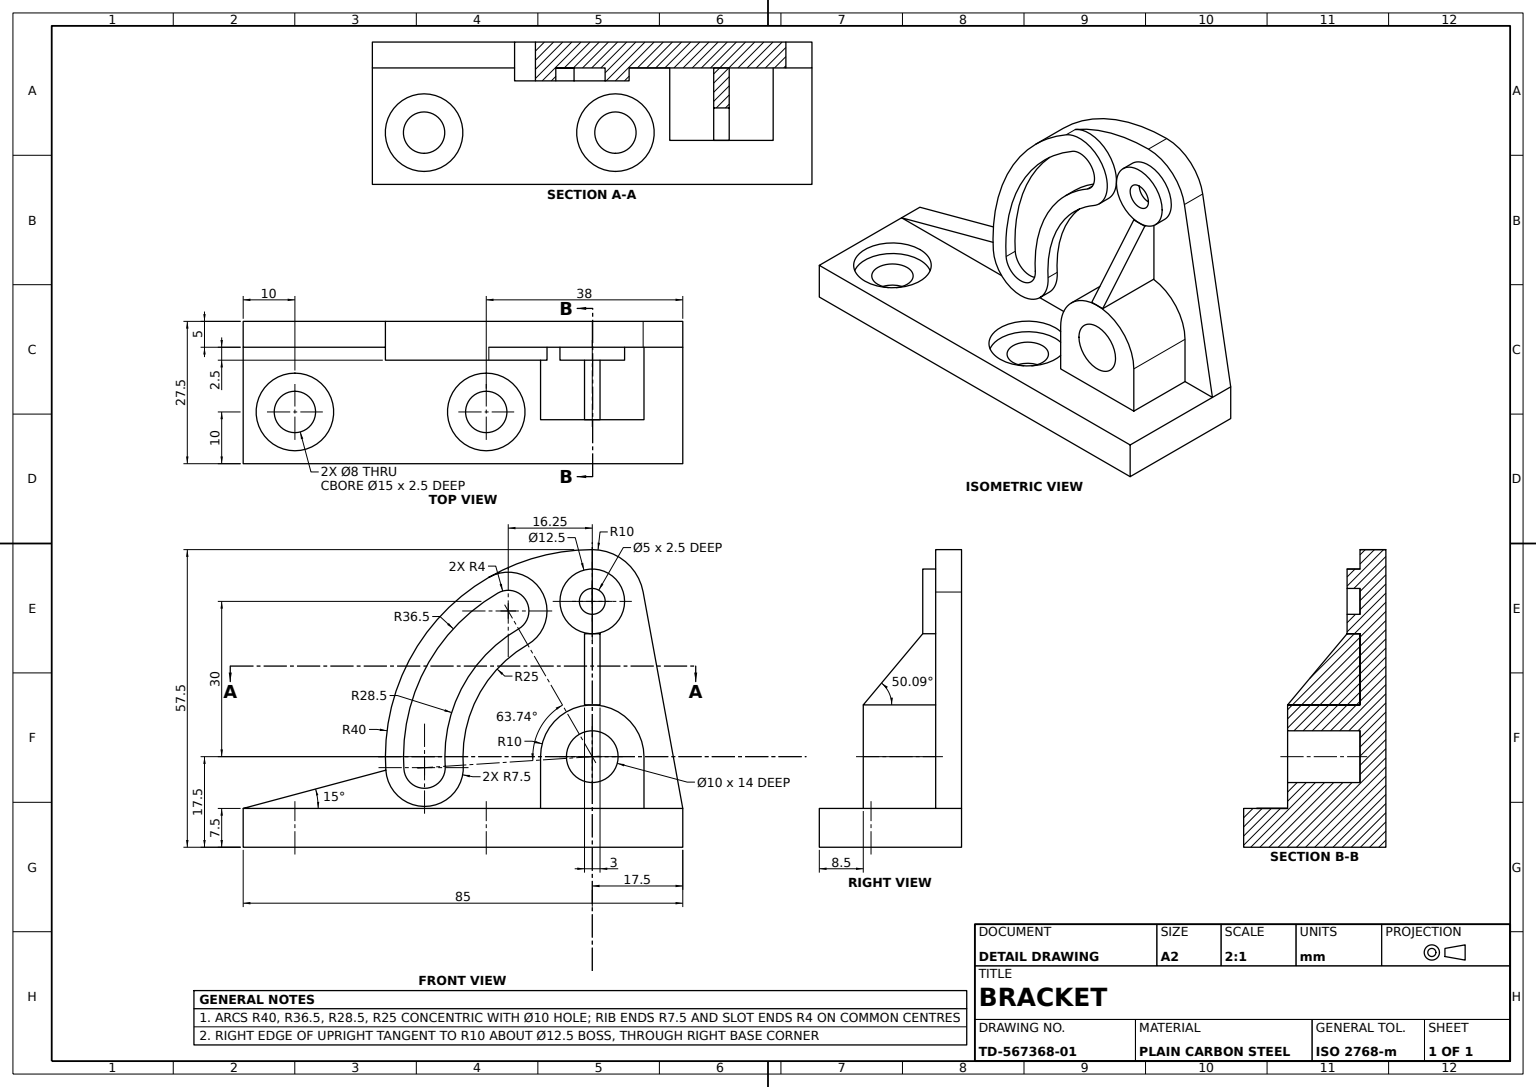
SolidWorks part; units mm, degrees
material "Plain Carbon Steel"
ref_plane "Front Plane" through (0, 0, 0) normal (0, 0, 1) x (1, 0, 0)
ref_plane "Top Plane" through (0, 0, 0) normal (0, 1, 0) x (1, 0, 0)
ref_plane "Right Plane" through (0, 0, 0) normal (1, 0, 0) x (0, 0, -1)
sketch "Base Plate Sketch" plane through (0, 0, 0) normal (0, 1, 0) x (1, 0, 0)
  line L1 (-42.5, -13.75) -> (42.5, -13.75)
  line L2 (-42.5, -13.75) -> (-42.5, 13.75)
  line L3 (-42.5, 13.75) -> (42.5, 13.75)
  line L4 (42.5, -13.75) -> (42.5, 13.75)
  line L5 (-42.5, -13.75) -> (42.5, 13.75) construction
  line L6 (-42.5, 13.75) -> (42.5, -13.75) construction
  point P0 (0, 0)
  dimension "D1" = 85
  dimension "D2" = 27.5
extrude "Base Plate" add sketch "Base Plate Sketch" along normal blind 7.5
sketch "Upright Profile Sketch" plane through (0, 0, -13.75) normal (0, 0, -1) x (-1, 0, 0)
  line L0 (-42.5, 7.5) -> (42.5, 7.5) construction
  line L1 (42.5, 7.5) -> (14.9149, 14.8914)
  line L2 (-34.8361, 49.3033) -> (-42.5, 7.5)
  line L3 (-42.5, 7.5) -> (42.5, 7.5)
  arc A0 (-25, 57.5) -> (-34.8361, 49.3033) centre (-25, 47.5) ccw
  arc A1 (-25, 57.5) -> (14.9149, 14.8914) centre (-25, 17.5) cw
  dimension "D1" = 20
  dimension "D4" = 40
  dimension "D2" = 40
  dimension "D3" = 17.5
  dimension "D5" = 15
extrude "Upright" add sketch "Upright Profile Sketch" against normal blind 5
sketch "Upright Rim Boss Sketch" plane through (0, 0, -8.75) normal (0, 0, 1) x (1, 0, 0)
  circle A0 centre (25, 47.5) radius 6.25
  circle A1 centre (25, 47.5) radius 2.5
  dimension "D1" = 12.5
  dimension "D2" = 5
extrude "Upright Rim Boss" add sketch "Upright Rim Boss Sketch" along normal blind 2.5
sketch "Bushing Block Sketch" plane through (0, 0, -8.75) normal (0, 0, 1) x (1, 0, 0)
  line L0 (42.5, 7.5) -> (-42.5, 7.5) construction
  line L1 (15, 17.5) -> (15, 7.5)
  line L2 (15, 7.5) -> (35, 7.5)
  line L3 (35, 7.5) -> (35, 17.5)
  arc A0 (35, 17.5) -> (15, 17.5) centre (25, 17.5) ccw
  circle A1 centre (25, 17.5) radius 5
  dimension "D1" = 20
  dimension "D2" = 10
  dimension "D3" = 17.5
  dimension "D4" = 10
extrude "Bushing Block" add sketch "Bushing Block Sketch" along normal blind 14
sketch "Counterbore Sketch 2xØ15" plane through (0, 7.5, 0) normal (0, 1, 0) x (1, 0, 0)
  line L0 (-42.5, -13.75) -> (42.5, -13.75) construction
  line L1 (42.5, -13.75) -> (42.5, 8.75) construction
  line L2 (-42.5, 8.75) -> (-42.5, -13.75) construction
  circle A0 centre (4.5, -3.75) radius 7.5
  circle A1 centre (-32.5, -3.75) radius 7.5
  dimension "D1" = 15
  dimension "D4" = 15
  dimension "D2" = 10
  dimension "D3" = 38
  dimension "D5" = 10
  dimension "D6" = 10
extrude "Counterbores 2xØ15" cut sketch "Counterbore Sketch 2xØ15" against normal blind 2.5
sketch "Mounting Hole Sketch 2xØ8" plane through (0, 5, 0) normal (0, 1, 0) x (1, 0, 0)
  circle A0 centre (-32.5, -3.75) radius 4
  circle A1 centre (4.5, -3.75) radius 4
  dimension "D1" = 8
  dimension "D2" = 8
extrude "Mounting Holes 2xØ8" cut sketch "Mounting Hole Sketch 2xØ8" against normal through all
ref_plane "Link Plate Plane" through (25, 0, 0) normal (1, 0, 0) x (0, 0, -1)
sketch "Link Plate Sketch" plane through (25, 0, 0) normal (1, 0, 0) x (0, 0, -1)
  line L0 (6.25, 41.25) -> (-5.25, 27.5)
  line L1 (6.25, 41.25) -> (8.75, 41.25)
  line L2 (8.75, 41.25) -> (8.75, 27.5)
  line L3 (8.75, 27.5) -> (-5.25, 27.5)
extrude "Link Plate" add sketch "Link Plate Sketch" along normal mid plane 3 separate body
sketch "Curved Guide Rib Sketch" plane through (0, 0, -8.75) normal (0, 0, 1) x (1, 0, 0)
  arc A0 (5, 52.141) -> (-14.9149, 14.8914) centre (25, 17.5) ccw
  arc A4 (12.5, 39.1506) -> (0.0532, 15.8696) centre (25, 17.5) ccw
  arc A5 (5, 52.141) -> (12.5, 39.1506) centre (8.75, 45.6458) cw
  arc A6 (-14.9149, 14.8914) -> (0.0532, 15.8696) centre (-7.4308, 15.3805) ccw
  arc A7 (8.75, 45.6458) -> (-7.4308, 15.3805) centre (25, 17.5) ccw construction
  arc A8 (6.75, 49.1099) -> (-11.4223, 15.1197) centre (25, 17.5) ccw
  arc A9 (10.75, 42.1817) -> (-3.4393, 15.6414) centre (25, 17.5) ccw
  arc A10 (10.75, 42.1817) -> (6.75, 49.1099) centre (8.75, 45.6458) ccw
  arc A11 (-11.4223, 15.1197) -> (-3.4393, 15.6414) centre (-7.4308, 15.3805) ccw
  point P5 (-3.661, 32.8231)
  dimension "D1" = 32.4308
  dimension "D2" = 4
  dimension "D3" = 28.661
  dimension "D4" = 12.8227
  dimension "D6" = 16.25
  dimension "D7" = 7.5
extrude "Curved Guide Rib" add sketch "Curved Guide Rib Sketch" along normal blind 2.5
